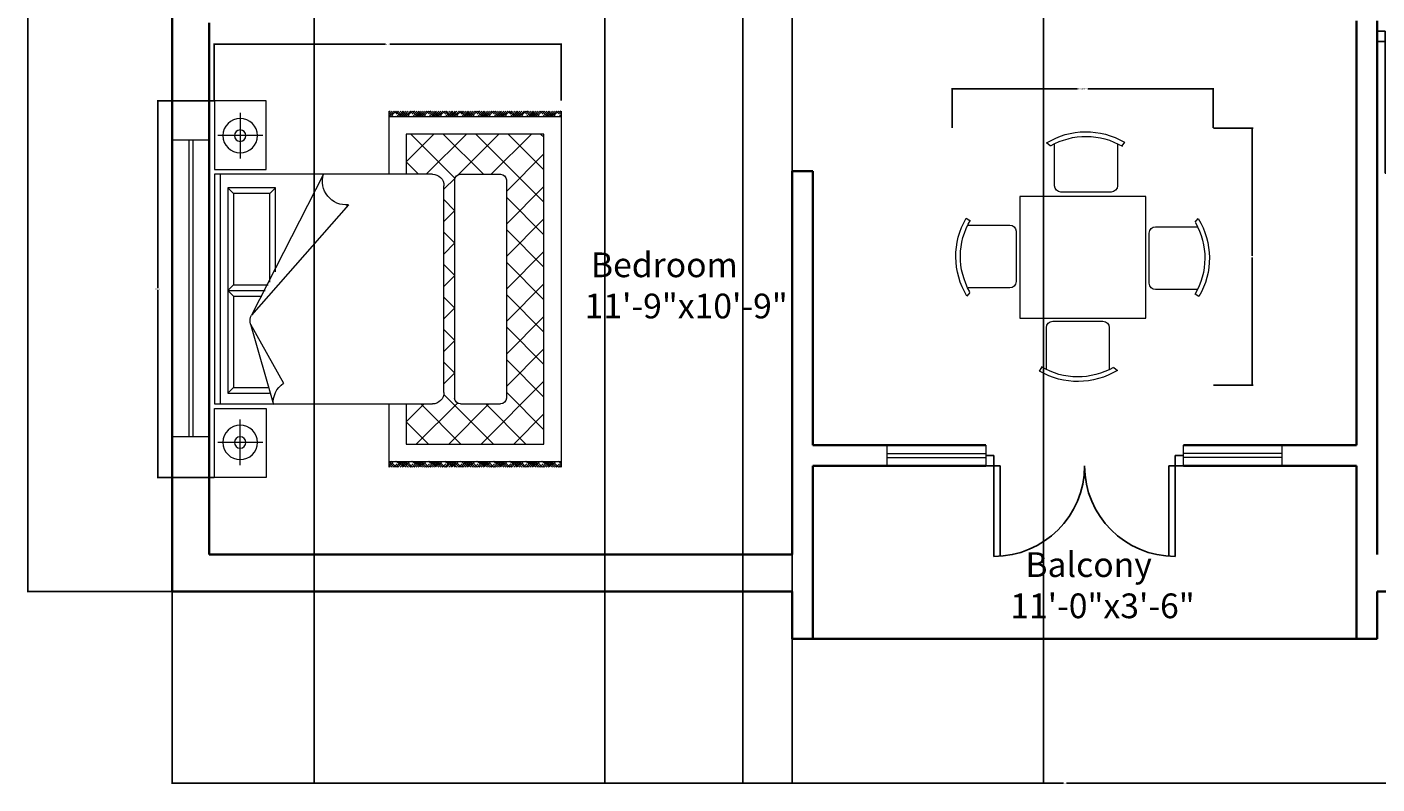
# Model space of a CAD drawing. Units: inches. Extents: x 3198 to 3702, y 1509 to 2253.
# Tile 1 of 6: x 3198 to 3526, y 1509 to 1693. Entities that reach past the tile are written whole.
import ezdxf

# ---------------------------------------------------------------- set-up
doc = ezdxf.new("R2010")
doc.units = ezdxf.units.IN
for name, color, linetype, lineweight in [('A-ANNO-DIMS', 2, 'Continuous', 18), ('A-AREA-IDEN', 7, 'Continuous', 18), ('A-DOOR', 3, 'Continuous', 25), ('A-FURN', 8, 'Continuous', 13), ('A-GLAZ', 4, 'Continuous', 18), ('A-WALL', 7, 'Continuous', 35)]:
    doc.layers.add(name, color=color, linetype=linetype, lineweight=lineweight)
doc.styles.get("Standard").update_dxf_attribs({"font": 'arial.ttf'})
doc.dimstyles.get("Standard").update_dxf_attribs({"dimtxt": 0.18, "dimasz": 0.18, "dimexe": 0.18, "dimexo": 0.0625, "dimgap": 0.09, "dimtad": 0, "dimtih": 1, "dimtoh": 1, "dimdec": 4, "dimzin": 0, "dimdsep": 46, "dimtxsty": 'Standard', "dimcen": 0.09, "dimadec": 0, "dimazin": 0, "dimtfac": 1, "dimtdec": 4, "dimtofl": 0, "dimtmove": 0, "dimatfit": 3, "dimfxl": 1, "dimtolj": 1, "dimtzin": 0, "dimarcsym": 0})

# ---------------------------------------------------------------- blocks, each defined once
blk = doc.blocks.new('A$C3E2236F0')
at = {"linetype": 'ByBlock'}
for p, q in [((0.639, 1.827), (0.658, 1.799)), ((0.692, 1.816), (0.692, 1.495)), ((1.172, 1.495), (1.172, 1.816)), ((1.207, 1.799), (1.235, 1.822)), ((0.74, 1.447), (1.124, 1.447)), ((0.489, 0.494), (0.489, 1.422)), ((0.489, 1.422), (1.452, 1.422)), ((1.452, 1.422), (1.452, 0.494)), ((0.108, 1.227), (0.085, 1.255)), ((1.857, 1.258), (1.829, 1.239)), ((0.412, 1.192), (0.091, 1.192)), ((0.46, 0.76), (0.46, 1.144)), ((1.477, 1.157), (1.477, 0.773)), ((1.846, 1.205), (1.525, 1.205)), ((1.525, 0.725), (1.846, 0.725)), ((0.08, 0.659), (0.108, 0.678)), ((0.091, 0.712), (0.412, 0.712)), ((1.829, 0.69), (1.852, 0.662)), ((1.452, 0.494), (0.489, 0.494)), ((1.187, 0.46), (0.803, 0.46)), ((0.755, 0.412), (0.755, 0.091)), ((1.235, 0.091), (1.235, 0.412)), ((0.72, 0.108), (0.692, 0.085)), ((1.288, 0.08), (1.269, 0.108))]:
    blk.add_line(p, q, dxfattribs=at)
for centre, radius, start, end in [((0.932, 1.328), 0.579, 58.5054, 120.4019), ((0.932, 1.328), 0.544, 60.0817, 120.6821), ((0.74, 1.495), 0.048, 180, 270), ((1.124, 1.495), 0.048, 270, 0), ((0.579, 0.952), 0.579, 148.5054, 210.4019), ((1.358, 0.965), 0.544, 330.0817, 30.6821), ((1.358, 0.965), 0.579, 328.5054, 30.4019), ((0.579, 0.952), 0.544, 150.0817, 210.6821), ((0.412, 1.144), 0.048, 0, 90), ((1.525, 1.157), 0.048, 90, 180), ((0.412, 0.76), 0.048, 270, 0), ((1.525, 0.773), 0.048, 180, 270), ((0.803, 0.412), 0.048, 90, 180), ((1.187, 0.412), 0.048, 0, 90), ((0.995, 0.579), 0.544, 240.0817, 300.6821), ((0.995, 0.579), 0.579, 238.5054, 300.4019)]:
    blk.add_arc(centre, radius, start, end, dxfattribs=at)
blk = doc.blocks.new('A$C4CB008C5')
for p, q in [((0, 3.019), (0.6, 3.019)), ((0, 2.569), (0, 3.019)), ((0.304, 2.6), (0.304, 2.992)), ((0.6, 3.019), (0.6, 2.569)), ((0.64, 1.121), (0.64, 3.021)), ((0.64, 3.021), (2.64, 3.021)), ((0.64, 2.971), (2.64, 2.971)), ((2.64, 3.021), (2.64, 1.121)), ((3.279, 3.019), (2.679, 3.019)), ((2.679, 3.019), (2.679, 2.569)), ((2.975, 2.6), (2.975, 2.992)), ((3.279, 2.569), (3.279, 3.019)), ((0.759, 2.905), (2.547, 2.905)), ((0.759, 2.489), (0.759, 2.905)), ((0.759, 2.905), (0.809, 2.855)), ((0.809, 2.855), (1.603, 2.855)), ((0.809, 2.539), (0.809, 2.855)), ((1.603, 2.855), (1.653, 2.905)), ((1.603, 2.855), (1.603, 2.551)), ((1.653, 2.905), (1.653, 2.579)), ((1.653, 2.905), (1.703, 2.855)), ((1.703, 2.855), (1.703, 2.607)), ((1.703, 2.855), (2.497, 2.855)), ((2.497, 2.855), (2.547, 2.905)), ((2.497, 2.855), (2.497, 2.556)), ((2.547, 2.905), (2.547, 2.54)), ((0.106, 2.796), (0.503, 2.796)), ((1.946, 2.705), (2.646, 2.507)), ((1.946, 2.705), (2.46, 2.418)), ((3.174, 2.796), (2.776, 2.796)), ((0.64, 2.071), (1.866, 2.698)), ((0.906, 1.854), (1.866, 2.698)), ((0.6, 2.569), (0, 2.569)), ((0.809, 2.539), (0.759, 2.489)), ((1.49, 2.489), (0.759, 2.489)), ((1.58, 2.539), (0.809, 2.539)), ((2.679, 2.569), (3.279, 2.569)), ((0.907, 1.867), (0.919, 1.867)), ((0.09, 1.5), (0.64, 1.5)), ((0.09, 1.491), (0.099, 1.5)), ((0.09, 1.473), (0.116, 1.5)), ((0.09, 1.456), (0.134, 1.5)), ((0.09, 1.474), (0.09, 1.475)), ((0.09, 1.438), (0.126, 1.474)), ((0.117, 1.43), (0.09, 1.457)), ((0.14, 1.389), (0.09, 1.439)), ((0.09, 1.42), (0.099, 1.43)), ((0.14, 1.372), (0.09, 1.422)), ((0.09, 1.368), (0.14, 1.417)), ((0.14, 1.46), (0.108, 1.492)), ((0.117, 1.412), (0.14, 1.435)), ((0.14, 1.478), (0.118, 1.5)), ((0.14, 1.496), (0.135, 1.5)), ((0.14, 1.442), (0.135, 1.448)), ((0.14, 0), (0.14, 1.5)), ((2.64, 1.5), (3.19, 1.5)), ((3.14, 1.496), (3.144, 1.5)), ((3.14, 1.478), (3.162, 1.5)), ((3.14, 1.5), (3.14, 0)), ((3.14, 1.46), (3.171, 1.492)), ((3.14, 1.442), (3.145, 1.448)), ((3.14, 1.389), (3.19, 1.439)), ((3.162, 1.412), (3.14, 1.435)), ((3.14, 1.372), (3.19, 1.422)), ((3.189, 1.368), (3.14, 1.417)), ((3.19, 1.456), (3.145, 1.5)), ((3.19, 1.438), (3.154, 1.474)), ((3.162, 1.43), (3.19, 1.457)), ((3.19, 1.473), (3.163, 1.5)), ((3.19, 1.42), (3.18, 1.43)), ((3.19, 1.491), (3.181, 1.5)), ((3.189, 1.474), (3.19, 1.475)), ((0.14, 1.354), (0.09, 1.404)), ((0.09, 1.35), (0.14, 1.4)), ((0.14, 1.336), (0.09, 1.386)), ((0.09, 1.332), (0.14, 1.382)), ((0.09, 1.314), (0.14, 1.364)), ((0.09, 1.297), (0.126, 1.333)), ((0.09, 1.333), (0.09, 1.333)), ((0.117, 1.288), (0.09, 1.316)), ((0.14, 1.248), (0.09, 1.298)), ((0.14, 1.319), (0.108, 1.35)), ((0.117, 1.271), (0.14, 1.294)), ((0.14, 1.301), (0.135, 1.306)), ((0.29, 1.108), (0.532, 1.35)), ((0.29, 0.15), (0.29, 1.35)), ((0.29, 1.35), (0.64, 1.35)), ((0.674, 0.926), (0.29, 1.31)), ((0.64, 1.243), (0.533, 1.35)), ((2.64, 1.195), (2.795, 1.35)), ((2.64, 1.35), (2.99, 1.35)), ((2.99, 1.156), (2.795, 1.35)), ((2.99, 1.35), (2.99, 0.15)), ((3.14, 1.354), (3.19, 1.404)), ((3.19, 1.35), (3.14, 1.4)), ((3.14, 1.336), (3.19, 1.386)), ((3.19, 1.332), (3.14, 1.382)), ((3.19, 1.314), (3.14, 1.364)), ((3.14, 1.319), (3.171, 1.35)), ((3.14, 1.301), (3.145, 1.306)), ((3.14, 1.248), (3.19, 1.298)), ((3.162, 1.271), (3.14, 1.294)), ((3.19, 1.297), (3.154, 1.333)), ((3.162, 1.288), (3.19, 1.316)), ((3.189, 1.333), (3.19, 1.333)), ((0.09, 1.279), (0.099, 1.288)), ((0.14, 1.23), (0.09, 1.28)), ((0.09, 1.227), (0.14, 1.276)), ((0.14, 1.213), (0.09, 1.263)), ((0.09, 1.208), (0.14, 1.258)), ((0.14, 1.195), (0.09, 1.245)), ((0.09, 1.19), (0.14, 1.24)), ((0.09, 1.173), (0.14, 1.223)), ((0.09, 1.191), (0.09, 1.192)), ((0.09, 1.155), (0.126, 1.191)), ((0.14, 1.177), (0.108, 1.209)), ((2.632, 0.904), (2.99, 1.262)), ((2.99, 0.873), (2.64, 1.223)), ((3.14, 1.23), (3.19, 1.28)), ((3.189, 1.227), (3.14, 1.276)), ((3.14, 1.213), (3.19, 1.263)), ((3.19, 1.208), (3.14, 1.258)), ((3.14, 1.195), (3.19, 1.245)), ((3.19, 1.19), (3.14, 1.24)), ((3.19, 1.173), (3.14, 1.223)), ((3.14, 1.177), (3.171, 1.209)), ((3.19, 1.155), (3.154, 1.191)), ((3.19, 1.279), (3.18, 1.288)), ((3.189, 1.191), (3.19, 1.192)), ((0.117, 1.147), (0.09, 1.174)), ((0.14, 1.107), (0.09, 1.157)), ((0.09, 1.137), (0.099, 1.147)), ((0.14, 1.089), (0.09, 1.139)), ((0.09, 1.085), (0.14, 1.134)), ((0.14, 1.071), (0.09, 1.121)), ((0.09, 1.067), (0.14, 1.117)), ((0.14, 1.054), (0.09, 1.104)), ((0.09, 1.049), (0.14, 1.099)), ((0.09, 1.031), (0.14, 1.081)), ((0.14, 1.036), (0.108, 1.067)), ((0.117, 1.129), (0.14, 1.152)), ((0.14, 1.16), (0.135, 1.165)), ((0.29, 0.825), (0.64, 1.175)), ((3.14, 1.16), (3.145, 1.165)), ((3.14, 1.107), (3.19, 1.157)), ((3.162, 1.129), (3.14, 1.152)), ((3.14, 1.089), (3.19, 1.139)), ((3.189, 1.085), (3.14, 1.134)), ((3.14, 1.071), (3.19, 1.121)), ((3.19, 1.067), (3.14, 1.117)), ((3.14, 1.054), (3.19, 1.104)), ((3.19, 1.049), (3.14, 1.099)), ((3.19, 1.031), (3.14, 1.081)), ((3.14, 1.036), (3.171, 1.067)), ((3.162, 1.147), (3.19, 1.174)), ((3.19, 1.137), (3.18, 1.147)), ((0.09, 1.05), (0.09, 1.051)), ((0.09, 1.014), (0.126, 1.05)), ((0.117, 1.006), (0.09, 1.033)), ((0.14, 0.965), (0.09, 1.015)), ((0.09, 0.996), (0.099, 1.006)), ((0.14, 0.948), (0.09, 0.998)), ((0.09, 0.944), (0.14, 0.993)), ((0.14, 0.93), (0.09, 0.98)), ((0.09, 0.925), (0.14, 0.975)), ((0.14, 0.912), (0.09, 0.962)), ((0.09, 0.908), (0.14, 0.958)), ((0.117, 0.988), (0.14, 1.011)), ((0.14, 1.018), (0.135, 1.023)), ((0.64, 0.677), (0.29, 1.027)), ((0.673, 0.925), (0.769, 1.021)), ((2.54, 1.021), (0.74, 1.021)), ((0.955, 0.928), (0.861, 1.021)), ((0.959, 0.928), (1.052, 1.021)), ((1.238, 0.928), (1.144, 1.021)), ((1.241, 0.928), (1.335, 1.021)), ((1.52, 0.928), (1.427, 1.021)), ((1.524, 0.928), (1.618, 1.021)), ((1.803, 0.928), (1.71, 1.021)), ((1.807, 0.928), (1.9, 1.021)), ((2.086, 0.928), (1.993, 1.021)), ((2.09, 0.928), (2.183, 1.021)), ((2.369, 0.928), (2.276, 1.021)), ((2.373, 0.928), (2.466, 1.021)), ((2.99, 0.59), (2.557, 1.023)), ((2.64, 0.629), (2.99, 0.979)), ((3.14, 1.018), (3.145, 1.023)), ((3.14, 0.965), (3.19, 1.015)), ((3.162, 0.988), (3.14, 1.011)), ((3.14, 0.948), (3.19, 0.998)), ((3.189, 0.944), (3.14, 0.993)), ((3.14, 0.93), (3.19, 0.98)), ((3.19, 0.925), (3.14, 0.975)), ((3.14, 0.912), (3.19, 0.962)), ((3.19, 0.908), (3.14, 0.958)), ((3.19, 1.014), (3.154, 1.05)), ((3.162, 1.006), (3.19, 1.033)), ((3.19, 0.996), (3.18, 1.006)), ((3.189, 1.05), (3.19, 1.051)), ((0.09, 0.89), (0.14, 0.94)), ((0.09, 0.908), (0.09, 0.909)), ((0.09, 0.872), (0.126, 0.908)), ((0.117, 0.864), (0.09, 0.891)), ((0.14, 0.824), (0.09, 0.874)), ((0.09, 0.855), (0.099, 0.864)), ((0.14, 0.806), (0.09, 0.856)), ((0.09, 0.802), (0.14, 0.852)), ((0.14, 0.788), (0.09, 0.838)), ((0.09, 0.784), (0.14, 0.834)), ((0.14, 0.894), (0.108, 0.926)), ((0.117, 0.847), (0.14, 0.869)), ((0.14, 0.877), (0.135, 0.882)), ((0.29, 0.542), (0.643, 0.895)), ((0.64, 0.878), (0.64, 0.528)), ((0.69, 0.928), (2.59, 0.928)), ((2.64, 0.878), (2.64, 0.528)), ((3.19, 0.89), (3.14, 0.94)), ((3.14, 0.894), (3.171, 0.926)), ((3.14, 0.877), (3.145, 0.882)), ((3.14, 0.824), (3.19, 0.874)), ((3.162, 0.847), (3.14, 0.869)), ((3.14, 0.806), (3.19, 0.856)), ((3.189, 0.802), (3.14, 0.852)), ((3.14, 0.788), (3.19, 0.838)), ((3.19, 0.784), (3.14, 0.834)), ((3.19, 0.872), (3.154, 0.908)), ((3.162, 0.864), (3.19, 0.891)), ((3.19, 0.855), (3.18, 0.864)), ((3.189, 0.908), (3.19, 0.909)), ((0.14, 0.771), (0.09, 0.821)), ((0.09, 0.766), (0.14, 0.816)), ((0.09, 0.749), (0.14, 0.799)), ((0.09, 0.767), (0.09, 0.768)), ((0.09, 0.731), (0.126, 0.767)), ((0.117, 0.723), (0.09, 0.75)), ((0.14, 0.682), (0.09, 0.732)), ((0.09, 0.713), (0.099, 0.723)), ((0.14, 0.665), (0.09, 0.715)), ((0.09, 0.661), (0.14, 0.71)), ((0.14, 0.753), (0.108, 0.785)), ((0.117, 0.705), (0.14, 0.728)), ((0.14, 0.735), (0.135, 0.74)), ((0.884, 0.15), (0.29, 0.744)), ((3.14, 0.771), (3.19, 0.821)), ((3.19, 0.766), (3.14, 0.816)), ((3.19, 0.749), (3.14, 0.799)), ((3.14, 0.753), (3.171, 0.785)), ((3.14, 0.735), (3.145, 0.74)), ((3.14, 0.682), (3.19, 0.732)), ((3.162, 0.705), (3.14, 0.728)), ((3.14, 0.665), (3.19, 0.715)), ((3.189, 0.661), (3.14, 0.71)), ((3.19, 0.731), (3.154, 0.767)), ((3.162, 0.723), (3.19, 0.75)), ((3.19, 0.713), (3.18, 0.723)), ((3.189, 0.767), (3.19, 0.768)), ((0.14, 0.647), (0.09, 0.697)), ((0.09, 0.642), (0.14, 0.692)), ((0.14, 0.629), (0.09, 0.679)), ((0.09, 0.625), (0.14, 0.675)), ((0.09, 0.607), (0.14, 0.657)), ((0.09, 0.589), (0.126, 0.626)), ((0.09, 0.626), (0.09, 0.626)), ((0.117, 0.581), (0.09, 0.609)), ((0.14, 0.541), (0.09, 0.591)), ((0.14, 0.612), (0.108, 0.643)), ((0.14, 0.594), (0.135, 0.599)), ((0.29, 0.259), (0.64, 0.609)), ((2.443, 0.15), (2.99, 0.696)), ((2.99, 0.307), (2.64, 0.657)), ((3.14, 0.647), (3.19, 0.697)), ((3.19, 0.642), (3.14, 0.692)), ((3.14, 0.629), (3.19, 0.679)), ((3.19, 0.625), (3.14, 0.675)), ((3.19, 0.607), (3.14, 0.657)), ((3.14, 0.612), (3.171, 0.643)), ((3.14, 0.594), (3.145, 0.599)), ((3.14, 0.541), (3.19, 0.591)), ((3.19, 0.589), (3.154, 0.626)), ((3.162, 0.581), (3.19, 0.609)), ((3.189, 0.626), (3.19, 0.626)), ((0.09, 0.572), (0.099, 0.581)), ((0.14, 0.523), (0.09, 0.573)), ((0.09, 0.519), (0.14, 0.569)), ((0.14, 0.506), (0.09, 0.556)), ((0.09, 0.501), (0.14, 0.551)), ((0.14, 0.488), (0.09, 0.538)), ((0.09, 0.483), (0.14, 0.533)), ((0.09, 0.466), (0.14, 0.516)), ((0.09, 0.484), (0.09, 0.485)), ((0.09, 0.448), (0.126, 0.484)), ((0.14, 0.47), (0.108, 0.502)), ((0.117, 0.564), (0.14, 0.586)), ((0.463, 0.15), (0.791, 0.478)), ((0.69, 0.478), (2.59, 0.478)), ((0.746, 0.15), (1.074, 0.478)), ((1.167, 0.15), (0.839, 0.478)), ((1.029, 0.15), (1.357, 0.478)), ((1.45, 0.15), (1.122, 0.478)), ((1.312, 0.15), (1.64, 0.478)), ((1.733, 0.15), (1.405, 0.478)), ((1.595, 0.15), (1.923, 0.478)), ((2.016, 0.15), (1.688, 0.478)), ((1.878, 0.15), (2.206, 0.478)), ((2.298, 0.15), (1.97, 0.478)), ((2.16, 0.15), (2.488, 0.478)), ((2.581, 0.15), (2.253, 0.478)), ((2.864, 0.15), (2.536, 0.478)), ((3.162, 0.564), (3.14, 0.586)), ((3.14, 0.523), (3.19, 0.573)), ((3.189, 0.519), (3.14, 0.569)), ((3.14, 0.506), (3.19, 0.556)), ((3.19, 0.501), (3.14, 0.551)), ((3.14, 0.488), (3.19, 0.538)), ((3.19, 0.483), (3.14, 0.533)), ((3.19, 0.466), (3.14, 0.516)), ((3.14, 0.47), (3.171, 0.502)), ((3.19, 0.448), (3.154, 0.484)), ((3.19, 0.572), (3.18, 0.581)), ((3.189, 0.484), (3.19, 0.485)), ((0.117, 0.44), (0.09, 0.467)), ((0.14, 0.399), (0.09, 0.449)), ((0.09, 0.43), (0.099, 0.44)), ((0.14, 0.382), (0.09, 0.432)), ((0.09, 0.378), (0.14, 0.427)), ((0.14, 0.364), (0.09, 0.414)), ((0.09, 0.36), (0.14, 0.41)), ((0.14, 0.346), (0.09, 0.396)), ((0.09, 0.342), (0.14, 0.392)), ((0.09, 0.324), (0.14, 0.374)), ((0.14, 0.329), (0.108, 0.36)), ((0.117, 0.422), (0.14, 0.445)), ((0.14, 0.453), (0.135, 0.458)), ((0.601, 0.15), (0.29, 0.462)), ((2.726, 0.15), (2.99, 0.414)), ((3.14, 0.453), (3.145, 0.458)), ((3.14, 0.399), (3.19, 0.449)), ((3.162, 0.422), (3.14, 0.445)), ((3.14, 0.382), (3.19, 0.432)), ((3.189, 0.378), (3.14, 0.427)), ((3.14, 0.364), (3.19, 0.414)), ((3.19, 0.36), (3.14, 0.41)), ((3.14, 0.346), (3.19, 0.396)), ((3.19, 0.342), (3.14, 0.392)), ((3.19, 0.324), (3.14, 0.374)), ((3.14, 0.329), (3.171, 0.36)), ((3.162, 0.44), (3.19, 0.467)), ((3.19, 0.43), (3.18, 0.44)), ((0.09, 0.307), (0.126, 0.343)), ((0.09, 0.343), (0.09, 0.343)), ((0.117, 0.299), (0.09, 0.326)), ((0.14, 0.258), (0.09, 0.308)), ((0.09, 0.289), (0.099, 0.299)), ((0.14, 0.24), (0.09, 0.29)), ((0.09, 0.237), (0.14, 0.286)), ((0.14, 0.223), (0.09, 0.273)), ((0.09, 0.218), (0.14, 0.268)), ((0.14, 0.205), (0.09, 0.255)), ((0.09, 0.201), (0.14, 0.251)), ((0.117, 0.281), (0.14, 0.304)), ((0.14, 0.311), (0.135, 0.316)), ((3.14, 0.311), (3.145, 0.316)), ((3.14, 0.258), (3.19, 0.308)), ((3.162, 0.281), (3.14, 0.304)), ((3.14, 0.24), (3.19, 0.29)), ((3.189, 0.237), (3.14, 0.286)), ((3.14, 0.223), (3.19, 0.273)), ((3.19, 0.218), (3.14, 0.268)), ((3.14, 0.205), (3.19, 0.255)), ((3.19, 0.201), (3.14, 0.251)), ((3.19, 0.307), (3.154, 0.343)), ((3.162, 0.299), (3.19, 0.326)), ((3.19, 0.289), (3.18, 0.299)), ((3.189, 0.343), (3.19, 0.343)), ((0.09, 0.183), (0.14, 0.233)), ((0.09, 0.201), (0.09, 0.202)), ((0.09, 0.165), (0.126, 0.201)), ((0.117, 0.157), (0.09, 0.184)), ((0.14, 0.117), (0.09, 0.167)), ((0.09, 0.148), (0.099, 0.157)), ((0.14, 0.099), (0.09, 0.149)), ((0.09, 0.095), (0.14, 0.144)), ((0.14, 0.081), (0.09, 0.131)), ((0.09, 0.077), (0.14, 0.127)), ((0.14, 0.187), (0.108, 0.219)), ((0.117, 0.139), (0.14, 0.162)), ((0.14, 0.17), (0.135, 0.175)), ((0.318, 0.15), (0.29, 0.179)), ((2.99, 0.15), (0.29, 0.15)), ((3.19, 0.183), (3.14, 0.233)), ((3.14, 0.187), (3.171, 0.219)), ((3.14, 0.17), (3.145, 0.175)), ((3.14, 0.117), (3.19, 0.167)), ((3.162, 0.139), (3.14, 0.162)), ((3.14, 0.099), (3.19, 0.149)), ((3.189, 0.095), (3.14, 0.144)), ((3.14, 0.081), (3.19, 0.131)), ((3.19, 0.077), (3.14, 0.127)), ((3.19, 0.165), (3.154, 0.201)), ((3.162, 0.157), (3.19, 0.184)), ((3.19, 0.148), (3.18, 0.157)), ((3.189, 0.201), (3.19, 0.202)), ((0.14, 0.064), (0.09, 0.114)), ((0.09, 0.059), (0.14, 0.109)), ((0.09, 0.041), (0.14, 0.091)), ((0.09, 0.06), (0.09, 0.061)), ((0.09, 0.024), (0.126, 0.06)), ((0.117, 0.016), (0.09, 0.043)), ((0.115, 0), (0.09, 0.025)), ((0.09, 0.006), (0.099, 0.016)), ((0.097, 0), (0.09, 0.008)), ((0.14, 0.046), (0.108, 0.078)), ((0.119, 0), (0.14, 0.021)), ((0.14, 0.028), (0.135, 0.033)), ((0.137, 0), (0.14, 0.003)), ((3.14, 0.064), (3.19, 0.114)), ((3.19, 0.059), (3.14, 0.109)), ((3.19, 0.041), (3.14, 0.091)), ((3.14, 0.046), (3.171, 0.078)), ((3.14, 0.028), (3.145, 0.033)), ((3.16, 0), (3.14, 0.021)), ((3.143, 0), (3.14, 0.003)), ((3.19, 0.024), (3.154, 0.06)), ((3.162, 0.016), (3.19, 0.043)), ((3.164, 0), (3.19, 0.025)), ((3.19, 0.006), (3.18, 0.016)), ((3.182, 0), (3.19, 0.008)), ((3.189, 0.06), (3.19, 0.061)), ((0.09, 0), (3.19, 0))]:
    blk.add_line(p, q)
for centre, radius in [((0.304, 2.796), 0.15), ((2.975, 2.796), 0.15), ((0.304, 2.796), 0.05), ((2.975, 2.796), 0.05)]:
    blk.add_circle(centre, radius)
for centre, radius, start, end in [((1.915, 2.61), 0.1, 71.7215, 119.0799), ((2.626, 2.31), 0.198, 84.1725, 146.9889), ((0.7, 1.873), 0.207, 354.6422, 106.9775), ((0.74, 1.121), 0.1, 180, 270), ((2.54, 1.121), 0.1, 270, 0), ((0.69, 0.878), 0.05, 90, 180), ((2.59, 0.878), 0.05, 0, 90), ((0.69, 0.528), 0.05, 180, 270), ((2.59, 0.528), 0.05, 270, 0)]:
    blk.add_arc(centre, radius, start, end)
blk = doc.blocks.new('DOOR-SINGLE-32')
for p, q in [((0, 34), (32, 34)), ((32, 36), (32, 34)), ((32, 34), (34.5, 34)), ((32, 32.5), (32, 34)), ((34.5, 34), (34.5, 36)), ((0.04, 32.5), (32, 32.5)), ((32, 0), (32, 2)), ((32, 2), (34.5, 2)), ((34.5, 2), (34.5, 0))]:
    blk.add_line(p, q)
blk.add_arc((32, 34), 32, 180, 270)
blk = doc.blocks.new('DOOR-BALCONY-PAIR-44')
for p, q in [((2, 2.5), (2, 24.5)), ((3.5, 2.5), (3.5, 24.45)), ((44.5, 2.5), (44.5, 24.45)), ((46, 2.5), (46, 24.5)), ((2, 2.5), (0, 2.5)), ((0, 0), (2, 0)), ((2, 0), (2, 2.5)), ((2, 2.5), (3.5, 2.5)), ((44.5, 2.5), (46, 2.5)), ((46, 0), (46, 2.5)), ((46, 2.5), (48, 2.5)), ((48, 0), (46, 0))]:
    blk.add_line(p, q)
for centre, start, end in [((2, 2.5), 0, 90), ((46, 2.5), 90, 180)]:
    blk.add_arc(centre, 22, start, end)
blk = doc.blocks.new('WIN-72-W9')
for p, q in [((0, 0), (0, 9)), ((72, 0), (72, 9)), ((72, 5), (0, 5)), ((72, 4), (0, 4))]:
    blk.add_line(p, q)
blk = doc.blocks.new('WIN-SIDELIGHT-24')
for p, q in [((0, 5), (0, 0)), ((24, 5), (24, 0)), ((0, 3), (24, 3)), ((0, 2), (24, 2))]:
    blk.add_line(p, q)
blk = doc.blocks.new('*D19')
at = {"layer": 'A-ANNO-DIMS', "color": 0, "lineweight": -2, "transparency": 16777216}
for p, q in [((3243.21, 1674.99), (3229.38, 1674.99)), ((3229.56, 1674.81), (3229.56, 1629.47)), ((3229.56, 1583.76), (3229.56, 1629.1)), ((3243.21, 1583.58), (3229.38, 1583.58))]:
    blk.add_line(p, q, dxfattribs=at)
at = {"layer": 'A-ANNO-DIMS', "color": 0, "transparency": 16777216}
for points in [[(3229.53, 1674.81), (3229.59, 1674.81), (3229.56, 1674.99)], [(3229.53, 1583.76), (3229.59, 1583.76), (3229.56, 1583.58)]]:
    blk.add_solid(points, dxfattribs=at)
at = {"layer": 'Defpoints', "color": 0, "transparency": 16777216}
for p in [(3243.27, 1674.99), (3229.56, 1583.58), (3243.27, 1583.58)]:
    blk.add_point(p, dxfattribs=at)
at = {"layer": 'A-ANNO-DIMS', "color": 0, "transparency": 16777216, "insert": (3229.56, 1629.28), "char_height": 0.18, "attachment_point": 5}
blk.add_mtext('\\A1;BED 91 TYP.', dxfattribs=at)
blk = doc.blocks.new('*D20')
at = {"layer": 'A-ANNO-DIMS', "color": 0, "lineweight": -2, "transparency": 16777216}
for p, q in [((3243.27, 1675.05), (3243.27, 1688.88)), ((3243.45, 1688.7), (3284.85, 1688.7)), ((3327.31, 1688.7), (3285.91, 1688.7)), ((3327.49, 1675.05), (3327.49, 1688.88))]:
    blk.add_line(p, q, dxfattribs=at)
at = {"layer": 'A-ANNO-DIMS', "color": 0, "transparency": 16777216}
for points in [[(3243.45, 1688.73), (3243.45, 1688.67), (3243.27, 1688.7)], [(3327.31, 1688.73), (3327.31, 1688.67), (3327.49, 1688.7)]]:
    blk.add_solid(points, dxfattribs=at)
at = {"layer": 'Defpoints', "color": 0, "transparency": 16777216}
for p in [(3243.27, 1688.7), (3243.27, 1674.99), (3327.49, 1674.99)]:
    blk.add_point(p, dxfattribs=at)
at = {"layer": 'A-ANNO-DIMS', "color": 0, "transparency": 16777216, "insert": (3285.38, 1688.7), "char_height": 0.18, "attachment_point": 5}
blk.add_mtext('\\A1;84 TYP.', dxfattribs=at)
blk = doc.blocks.new('*D29')
at = {"layer": 'A-ANNO-DIMS', "color": 0, "lineweight": -2, "transparency": 16777216}
for p, q in [((3422.38, 1668.43), (3422.38, 1678.06)), ((3422.56, 1677.88), (3452.8, 1677.88)), ((3485.59, 1677.88), (3455.35, 1677.88)), ((3485.77, 1668.43), (3485.77, 1678.06))]:
    blk.add_line(p, q, dxfattribs=at)
at = {"layer": 'A-ANNO-DIMS', "color": 0, "transparency": 16777216}
for points in [[(3422.56, 1677.91), (3422.56, 1677.85), (3422.38, 1677.88)], [(3485.59, 1677.91), (3485.59, 1677.85), (3485.77, 1677.88)]]:
    blk.add_solid(points, dxfattribs=at)
at = {"layer": 'Defpoints', "color": 0, "transparency": 16777216}
for p in [(3485.77, 1677.88), (3422.38, 1668.37), (3485.77, 1668.37)]:
    blk.add_point(p, dxfattribs=at)
at = {"layer": 'A-ANNO-DIMS', "color": 0, "transparency": 16777216, "insert": (3454.07, 1677.88), "char_height": 0.18, "attachment_point": 5}
blk.add_mtext('\\A1;DINING SET 63 TYP.', dxfattribs=at)
blk = doc.blocks.new('*D30')
at = {"layer": 'A-ANNO-DIMS', "color": 0, "lineweight": -2, "transparency": 16777216}
for p, q in [((3485.83, 1668.37), (3495.45, 1668.37)), ((3495.27, 1668.19), (3495.27, 1637.33)), ((3495.27, 1606.12), (3495.27, 1636.97)), ((3485.83, 1605.94), (3495.45, 1605.94))]:
    blk.add_line(p, q, dxfattribs=at)
at = {"layer": 'A-ANNO-DIMS', "color": 0, "transparency": 16777216}
for points in [[(3495.24, 1668.19), (3495.3, 1668.19), (3495.27, 1668.37)], [(3495.24, 1606.12), (3495.3, 1606.12), (3495.27, 1605.94)]]:
    blk.add_solid(points, dxfattribs=at)
at = {"layer": 'Defpoints', "color": 0, "transparency": 16777216}
for p in [(3485.77, 1668.37), (3485.77, 1605.94), (3495.27, 1605.94)]:
    blk.add_point(p, dxfattribs=at)
at = {"layer": 'A-ANNO-DIMS', "color": 0, "transparency": 16777216, "insert": (3495.27, 1637.15), "char_height": 0.18, "attachment_point": 5}
blk.add_mtext('\\A1;62 TYP.', dxfattribs=at)
blk = doc.blocks.new('*D43')
at = {"layer": 'A-ANNO-DIMS', "color": 0, "lineweight": -2, "transparency": 16777216}
for p, q in [((3233.05, 1555.83), (3233.05, 1509.16)), ((3666.55, 1555.83), (3666.55, 1509.16)), ((3233.23, 1509.34), (3449.4, 1509.34)), ((3666.37, 1509.34), (3450.2, 1509.34))]:
    blk.add_line(p, q, dxfattribs=at)
at = {"layer": 'A-ANNO-DIMS', "color": 0, "transparency": 16777216}
for points in [[(3233.23, 1509.37), (3233.23, 1509.31), (3233.05, 1509.34)], [(3666.37, 1509.37), (3666.37, 1509.31), (3666.55, 1509.34)]]:
    blk.add_solid(points, dxfattribs=at)
at = {"layer": 'Defpoints', "color": 0, "transparency": 16777216}
for p in [(3233.05, 1555.89), (3666.55, 1555.89), (3666.55, 1509.34)]:
    blk.add_point(p, dxfattribs=at)
at = {"layer": 'A-ANNO-DIMS', "color": 0, "transparency": 16777216, "insert": (3449.8, 1509.34), "char_height": 0.18, "attachment_point": 5}
blk.add_mtext('\\A1;433.5', dxfattribs=at)
blk = doc.blocks.new('*D50')
at = {"layer": 'A-ANNO-DIMS', "color": 0, "lineweight": -2, "transparency": 16777216}
for p, q in [((3232.98, 1844.89), (3197.82, 1844.89)), ((3198, 1844.71), (3198, 1700.57)), ((3198, 1556.07), (3198, 1700.21)), ((3232.98, 1555.89), (3197.82, 1555.89))]:
    blk.add_line(p, q, dxfattribs=at)
at = {"layer": 'A-ANNO-DIMS', "color": 0, "transparency": 16777216}
for points in [[(3197.97, 1844.71), (3198.03, 1844.71), (3198, 1844.89)], [(3197.97, 1556.07), (3198.03, 1556.07), (3198, 1555.89)]]:
    blk.add_solid(points, dxfattribs=at)
at = {"layer": 'Defpoints', "color": 0, "transparency": 16777216}
for p in [(3233.05, 1844.89), (3198, 1555.89), (3233.05, 1555.89)]:
    blk.add_point(p, dxfattribs=at)
at = {"layer": 'A-ANNO-DIMS', "color": 0, "transparency": 16777216, "insert": (3198, 1700.39), "char_height": 0.18, "attachment_point": 5}
blk.add_mtext('\\A1;289', dxfattribs=at)
blk = doc.blocks.new('*D51')
at = {"layer": 'A-ANNO-DIMS', "color": 0, "lineweight": -2, "transparency": 16777216}
for p, q in [((3267.55, 1844.83), (3267.55, 1509.16)), ((3383.55, 1844.83), (3383.55, 1509.16)), ((3267.73, 1509.34), (3325.27, 1509.34)), ((3383.37, 1509.34), (3325.83, 1509.34))]:
    blk.add_line(p, q, dxfattribs=at)
at = {"layer": 'A-ANNO-DIMS', "color": 0, "transparency": 16777216}
for points in [[(3267.73, 1509.37), (3267.73, 1509.31), (3267.55, 1509.34)], [(3383.37, 1509.37), (3383.37, 1509.31), (3383.55, 1509.34)]]:
    blk.add_solid(points, dxfattribs=at)
at = {"layer": 'Defpoints', "color": 0, "transparency": 16777216}
for p in [(3267.55, 1844.89), (3383.55, 1844.89), (3383.55, 1509.34)]:
    blk.add_point(p, dxfattribs=at)
at = {"layer": 'A-ANNO-DIMS', "color": 0, "transparency": 16777216, "insert": (3325.55, 1509.34), "char_height": 0.18, "attachment_point": 5}
blk.add_mtext('\\A1;116', dxfattribs=at)
blk = doc.blocks.new('*D52')
at = {"layer": 'A-ANNO-DIMS', "color": 0, "lineweight": -2, "transparency": 16777216}
for p, q in [((3383.55, 1844.83), (3383.55, 1509.16)), ((3444.55, 1844.83), (3444.55, 1509.16)), ((3383.73, 1509.34), (3413.85, 1509.34)), ((3444.37, 1509.34), (3414.25, 1509.34))]:
    blk.add_line(p, q, dxfattribs=at)
at = {"layer": 'A-ANNO-DIMS', "color": 0, "transparency": 16777216}
for points in [[(3383.73, 1509.37), (3383.73, 1509.31), (3383.55, 1509.34)], [(3444.37, 1509.37), (3444.37, 1509.31), (3444.55, 1509.34)]]:
    blk.add_solid(points, dxfattribs=at)
at = {"layer": 'Defpoints', "color": 0, "transparency": 16777216}
for p in [(3383.55, 1844.89), (3444.55, 1844.89), (3444.55, 1509.34)]:
    blk.add_point(p, dxfattribs=at)
at = {"layer": 'A-ANNO-DIMS', "color": 0, "transparency": 16777216, "insert": (3414.05, 1509.34), "char_height": 0.18, "attachment_point": 5}
blk.add_mtext('\\A1;61', dxfattribs=at)
blk = doc.blocks.new('*D57')
at = {"layer": 'A-ANNO-DIMS', "color": 0, "lineweight": -2, "transparency": 16777216}
for p, q in [((3338.05, 1698.83), (3338.05, 1509.16)), ((3383.55, 1698.83), (3383.55, 1509.16)), ((3338.23, 1509.34), (3360.47, 1509.34)), ((3383.37, 1509.34), (3361.13, 1509.34))]:
    blk.add_line(p, q, dxfattribs=at)
at = {"layer": 'A-ANNO-DIMS', "color": 0, "transparency": 16777216}
for points in [[(3338.23, 1509.37), (3338.23, 1509.31), (3338.05, 1509.34)], [(3383.37, 1509.37), (3383.37, 1509.31), (3383.55, 1509.34)]]:
    blk.add_solid(points, dxfattribs=at)
at = {"layer": 'Defpoints', "color": 0, "transparency": 16777216}
for p in [(3338.05, 1698.89), (3383.55, 1698.89), (3383.55, 1509.34)]:
    blk.add_point(p, dxfattribs=at)
at = {"layer": 'A-ANNO-DIMS', "color": 0, "transparency": 16777216, "insert": (3360.8, 1509.34), "char_height": 0.18, "attachment_point": 5}
blk.add_mtext('\\A1;45.5', dxfattribs=at)
blk = doc.blocks.new('*D60')
at = {"layer": 'A-ANNO-DIMS', "color": 0, "lineweight": -2, "transparency": 16777216}
for p, q in [((3371.55, 1792.83), (3371.55, 1509.16)), ((3383.55, 1792.83), (3383.55, 1509.16)), ((3371.73, 1509.34), (3377.34, 1509.34)), ((3383.37, 1509.34), (3377.76, 1509.34))]:
    blk.add_line(p, q, dxfattribs=at)
at = {"layer": 'A-ANNO-DIMS', "color": 0, "transparency": 16777216}
for points in [[(3371.73, 1509.37), (3371.73, 1509.31), (3371.55, 1509.34)], [(3383.37, 1509.37), (3383.37, 1509.31), (3383.55, 1509.34)]]:
    blk.add_solid(points, dxfattribs=at)
at = {"layer": 'Defpoints', "color": 0, "transparency": 16777216}
for p in [(3371.55, 1792.89), (3383.55, 1792.89), (3383.55, 1509.34)]:
    blk.add_point(p, dxfattribs=at)
at = {"layer": 'A-ANNO-DIMS', "color": 0, "transparency": 16777216, "insert": (3377.55, 1509.34), "char_height": 0.18, "attachment_point": 5}
blk.add_mtext('\\A1;12', dxfattribs=at)

msp = doc.modelspace()

# ---------------------------------------------------------------- linework, layer by layer
at = {"layer": 'A-WALL'}
for p, q in [((3233.0475, 1844.888), (3233.0475, 1555.888)), ((3242.0475, 1693.888), (3242.0475, 1564.888)), ((3520.5475, 1694.388), (3520.5475, 1591.388)), ((3525.5475, 1694.388), (3525.5475, 1564.888)), ((3383.5475, 1657.888), (3388.5475, 1657.888)), ((3383.5475, 1657.888), (3383.5475, 1564.888)), ((3388.5475, 1657.888), (3388.5475, 1591.388)), ((3388.5475, 1591.388), (3430.5475, 1591.388)), ((3478.5475, 1591.388), (3520.5475, 1591.388)), ((3388.5475, 1586.388), (3430.5475, 1586.388)), ((3388.5475, 1586.388), (3388.5475, 1544.388)), ((3478.5475, 1586.388), (3520.5475, 1586.388)), ((3520.5475, 1586.388), (3520.5475, 1544.388)), ((3242.0475, 1564.888), (3383.5475, 1564.888)), ((3233.0475, 1555.888), (3383.5475, 1555.888)), ((3383.5475, 1555.888), (3383.5475, 1544.388)), ((3525.5475, 1555.888), (3666.5475, 1555.888)), ((3525.5475, 1555.888), (3525.5475, 1544.388)), ((3383.5475, 1544.388), (3525.5475, 1544.388))]:
    msp.add_line(p, q, dxfattribs=at)

# ---------------------------------------------------------------- block references
at = {"layer": 'A-DOOR'}
for name, p, rotation in [('DOOR-SINGLE-32', (3561.5475, 1657.3875), 89.99999999999909), ('DOOR-BALCONY-PAIR-44', (3478.5479, 1588.888), 180)]:
    msp.add_blockref(name, p, dxfattribs=dict(at, rotation=rotation))
at = {"layer": 'A-FURN'}
for name, p, xscale, yscale, zscale, rotation in [('A$C4CB008C5', (3327.4909, 1674.9921), -27.87562936897135, 27.87562936897135, 27.87562936897135, 90), ('A$C3E2236F0', (3423.2889, 1667.4602), -31.78702146954402, 31.78702146954402, 31.78702146954402, 180)]:
    msp.add_blockref(name, p, dxfattribs=dict(at, xscale=xscale, yscale=yscale, zscale=zscale, rotation=rotation))
at = {"layer": 'A-GLAZ'}
for name, p, rotation in [('WIN-72-W9', (3242.0475, 1593.3875), 89.99999999999923), ('WIN-SIDELIGHT-24', (3502.5479, 1591.388), 180)]:
    msp.add_blockref(name, p, dxfattribs=dict(at, rotation=rotation))
msp.add_blockref('WIN-SIDELIGHT-24', (3406.547, 1586.388), dxfattribs=at)

# ---------------------------------------------------------------- texts
at = {"layer": 'A-AREA-IDEN', "attachment_point": 1}
for s, width, insert, char_height in [('  {\\H2.4x;Bedroom\\P11\'-9"x10\'-9"}', 75.551815, (3333.171, 1638.1699), 2.5), ('  Balcony\\P11\'-0"x3\'-6"', 59.912118, (3436.5154, 1565.4037), 6)]:
    msp.add_mtext_dynamic_manual_height_columns(s, width=width, gutter_width=12.5, heights=[0], dxfattribs=dict(at, insert=insert, char_height=char_height))

# ---------------------------------------------------------------- dimensions: what is measured, and where the dimension line sits
at = {"layer": 'A-ANNO-DIMS'}
dim = msp.add_linear_dim(base=(3197.9975, 1555.888), p1=(3233.0475, 1844.888), p2=(3233.0475, 1555.888), angle=90, dimstyle='Standard', override={"dimdec": 0, "dimlfac": 1, "dimrnd": 0, "dimzin": 0, "dimdsep": 46, "dimlunit": 2}, dxfattribs=at)
dim.commit()
dim.dimension.update_dxf_attribs({"geometry": '*D50', "text_midpoint": (3197.9975, 1700.388)})
for base, p1, p2, override, picture, middle in [((3383.5475, 1509.338), (3267.5475, 1844.888), (3383.5475, 1844.888), {"dimdec": 0, "dimlfac": 1, "dimrnd": 0, "dimzin": 0, "dimdsep": 46, "dimlunit": 2}, '*D51', (3325.5475, 1509.338)), ((3444.5475, 1509.338), (3383.5475, 1844.888), (3444.5475, 1844.888), {"dimdec": 0, "dimlfac": 1, "dimrnd": 0, "dimzin": 0, "dimdsep": 46, "dimlunit": 2}, '*D52', (3414.0475, 1509.338)), ((3383.5475, 1509.338), (3371.5475, 1792.888), (3383.5475, 1792.888), {"dimdec": 0, "dimlfac": 1, "dimrnd": 0, "dimzin": 0, "dimdsep": 46, "dimlunit": 2}, '*D60', (3377.5475, 1509.338)), ((3383.5475, 1509.338), (3338.0475, 1698.888), (3383.5475, 1698.888), {"dimdec": 1, "dimlfac": 1, "dimrnd": 0, "dimzin": 0, "dimdsep": 46, "dimlunit": 2}, '*D57', (3360.7975, 1509.338)), ((3666.5475, 1509.338), (3233.0475, 1555.888), (3666.5475, 1555.888), {"dimdec": 1, "dimlfac": 1, "dimrnd": 0, "dimzin": 0, "dimdsep": 46, "dimlunit": 2}, '*D43', (3449.7975, 1509.338))]:
    dim = msp.add_linear_dim(base=base, p1=p1, p2=p2, dimstyle='Standard', override=override, dxfattribs=at)
    dim.commit()
    dim.dimension.update_dxf_attribs({"geometry": picture, "text_midpoint": middle})
for base, p1, p2, angle, text, picture, middle in [((3243.2709, 1688.7045), (3327.4909, 1674.9921), (3243.2709, 1674.9921), 180, '<> TYP.', '*D20', (3285.3809, 1688.7045)), ((3229.5585, 1583.5761), (3243.2709, 1674.9921), (3243.2709, 1583.5761), 270, 'BED <> TYP.', '*D19', (3229.5585, 1629.2841)), ((3495.273, 1605.9374), (3485.7654, 1668.3681), (3485.7654, 1605.9374), 270, '<> TYP.', '*D30', (3495.273, 1637.1527))]:
    dim = msp.add_linear_dim(base=base, p1=p1, p2=p2, angle=angle, text=text, dimstyle='Standard', override={"dimdec": 0, "dimlfac": 1, "dimrnd": 0, "dimzin": 0, "dimdsep": 46, "dimlunit": 2}, dxfattribs=at)
    dim.commit()
    dim.dimension.update_dxf_attribs({"geometry": picture, "text_midpoint": middle})
dim = msp.add_linear_dim(base=(3485.7654, 1677.8758), p1=(3422.381, 1668.3681), p2=(3485.7654, 1668.3681), text='DINING SET <> TYP.', dimstyle='Standard', override={"dimdec": 0, "dimlfac": 1, "dimrnd": 0, "dimzin": 0, "dimdsep": 46, "dimlunit": 2}, dxfattribs=at)
dim.commit()
dim.dimension.update_dxf_attribs({"geometry": '*D29', "text_midpoint": (3454.0732, 1677.8758)})

doc.saveas('drawing.dxf')
